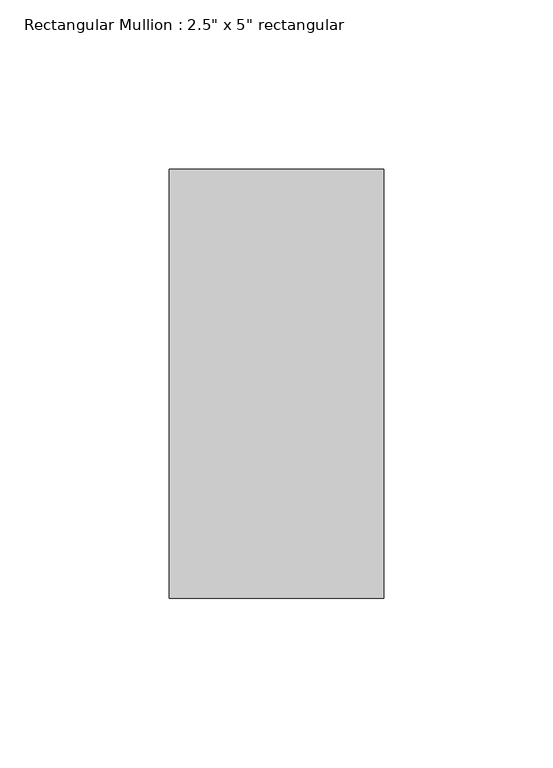
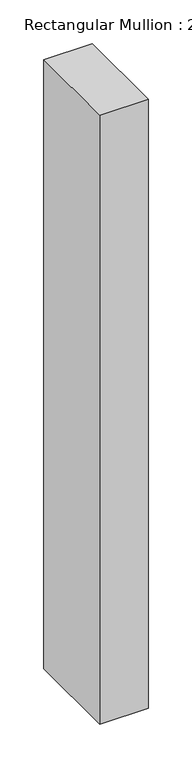
"""IFC4 building model written with IfcOpenShell, lengths in millimetres: member geometry."""

from ifc_helpers import new_model, si_unit, frame, origin, place, context, project, spatial, polyline, outline, extrude, source, transform, mapped, element, save


def member_62723634(model_context):
    return source(origin(), model_context, "Body", "SweptSolid", [
        extrude(outline(polyline([(0.0, 63.5), (0.0, -63.5), (-63.5, -63.5), (-63.5, 63.5), (0.0, 63.5)])), frame((0.0, 0.0, -845.8541168), z_axis=(0.0, 0.0, 1.0), x_axis=(1.0, 0.0, 0.0)), (0.0, 0.0, 1.0), 845.8541168),
    ])


if __name__ == "__main__":
    model = new_model("IFC4")
    model_context = context("Model", 3, world=origin())
    ifc_project = project(units=[si_unit("LENGTHUNIT", "METRE", prefix="MILLI")], contexts=[model_context])
    site = spatial("IfcSite", under=ifc_project)
    building = spatial("IfcBuilding", under=site)
    placement = place(None, origin())
    member_shape = member_62723634(model_context)
    element("IfcMember", 1, ObjectType="Rectangular Mullion : 2.5\" x 5\" rectangular", at=placement, inside=building, context=model_context, shape_type="MappedRepresentation", body=[
        mapped(member_shape, transform((0.0, 0.0, 0.0), x_axis=(1.0, 0.0, 0.0), y_axis=(0.0, 1.0, 0.0), z_axis=(0.0, 0.0, 1.0))),
    ])
    save(model, "model.ifc")

# Revit data of these elements
# Type "Rectangular Mullion : 2.5\" x 5\" rectangular"
#   built-in parameter 1007304 = 0.416667 (stored number, unit not read)
#   built-in parameter 1007301 = 0.104167 (stored number, unit not read)
#   built-in parameter 1007300 = 0.104167 (stored number, unit not read)
# Element 1 (IfcMember, "Rectangular Mullion : 2.5\" x 5\" rectangular")
#   Materials on its faces: "Aluminum"
# Materials
#   "Aluminum": class "Metal", colour RGB 247 247 247, transparency 0, Description = "Aluminum 6061", Cost = 0
